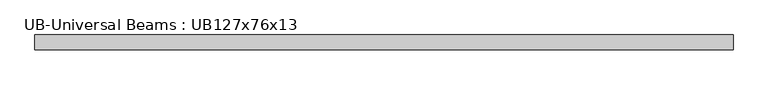
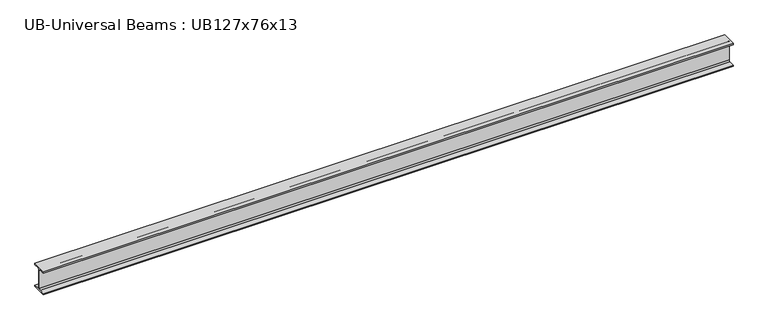
"""IFC4 building model written with IfcOpenShell, lengths in millimetres: member geometry, UB-Universal Beams : UB127x76x13."""

from ifc_helpers import new_model, si_unit, point, frame, frame_2d, origin, place, context, project, spatial, polyline, circle_curve, trimmed, segment, composite_curve, outline, extrude, source, transform, mapped, element, save


def ub_universal_beams_ub127x76x13_b97c8348(model_context):
    return source(origin(), model_context, "Body", "SweptSolid", [
        extrude(outline(composite_curve([segment(polyline([(38.0, -55.9), (38.0, -63.5), (-38.0, -63.5), (-38.0, -55.9), (-9.6, -55.9)]), True, "CONTINUOUS"), segment(trimmed(circle_curve(frame_2d((-9.6, -48.3)), 7.6), [point((-9.6, -55.9))], [point((-2.0, -48.3))], True, "CARTESIAN"), True, "CONTINUOUS"), segment(polyline([(-2.0, -48.3), (-2.0, 48.3)]), True, "CONTINUOUS"), segment(trimmed(circle_curve(frame_2d((-9.6, 48.3)), 7.6), [point((-2.0, 48.3))], [point((-9.6, 55.9))], True, "CARTESIAN"), True, "CONTINUOUS"), segment(polyline([(-9.6, 55.9), (-38.0, 55.9), (-38.0, 63.5), (38.0, 63.5), (38.0, 55.9), (9.6, 55.9)]), True, "CONTINUOUS"), segment(trimmed(circle_curve(frame_2d((9.6, 48.3)), 7.6), [point((9.6, 55.9))], [point((2.0, 48.3))], True, "CARTESIAN"), True, "CONTINUOUS"), segment(polyline([(2.0, 48.3), (2.0, -48.3)]), True, "CONTINUOUS"), segment(trimmed(circle_curve(frame_2d((9.6, -48.3)), 7.6), [point((2.0, -48.3))], [point((9.6, -55.9))], True, "CARTESIAN"), True, "CONTINUOUS"), segment(polyline([(9.6, -55.9), (38.0, -55.9)]), True, "CONTINUOUS")], self_intersect=False)), frame((-1575.05, 0.0, 0.0), z_axis=(1.0, 0.0, 0.0), x_axis=(0.0, 1.0, 0.0)), (0.0, 0.0, 1.0), 3575.0),
    ])


if __name__ == "__main__":
    model = new_model("IFC4")
    model_context = context("Model", 3, world=origin())
    ifc_project = project(units=[si_unit("LENGTHUNIT", "METRE", prefix="MILLI")], contexts=[model_context])
    site = spatial("IfcSite", under=ifc_project)
    building = spatial("IfcBuilding", under=site)
    placement = place(None, origin())
    ub_universal_beams_ub127x76x13_shape = ub_universal_beams_ub127x76x13_b97c8348(model_context)
    element("IfcMember", 1, ObjectType="UB-Universal Beams : UB127x76x13", at=placement, inside=building, context=model_context, shape_type="MappedRepresentation", body=[
        mapped(ub_universal_beams_ub127x76x13_shape, transform((0.0, 0.0, 0.0), x_axis=(1.0, 0.0, 0.0), y_axis=(0.0, 1.0, 0.0), z_axis=(0.0, 0.0, 1.0))),
    ])
    save(model, "model.ifc")

# Revit data of these elements
# Type "UB-Universal Beams : UB127x76x13"
#   Section Name Key = "UB127X76X13"
#   Width = 7.6 cm
#   Web Thickness = 0.4 cm
#   Web Fillet = 0.76 cm
#   Warping Constant = 2000.0 cm⁶
#   Torsional Moment of Inertia = 2.85 cm⁴
#   Section Area = 16.5 cm²
#   Plastic Modulus weak axis = 22.6 cm³
#   Plastic Modulus strong axis = 84.2 cm³
#   Nominal Weight = 13.00 kgf/m
#   Moment of Inertia weak axis = 55.70 cm⁴
#   Moment of Inertia strong axis = 473.00 cm⁴
#   Height = 12.7 cm
#   Flange Thickness = 0.76 cm
#   Elastic Modulus weak axis = 14.7 cm³
#   Elastic Modulus strong axis = 74.6 cm³
#   Centroid Vertical = 6.35 cm
#   Centroid Horizontal = 3.8 cm
#   Bolt Spacing = 4.0 cm
#   Length [instance default] = 1.5 m
#   Structural Material [instance default] = Metal - Steel 43-275
#   Type Comments = ""
#   Assembly Code = ""
# Element 1 (IfcMember, "UB-Universal Beams : UB127x76x13")
#   Materials on its faces: "Metal - Steel 43-275"
# Materials
#   "Metal - Steel 43-275": class "Metal", colour RGB 247 247 247, transparency 0, Cost = 0
